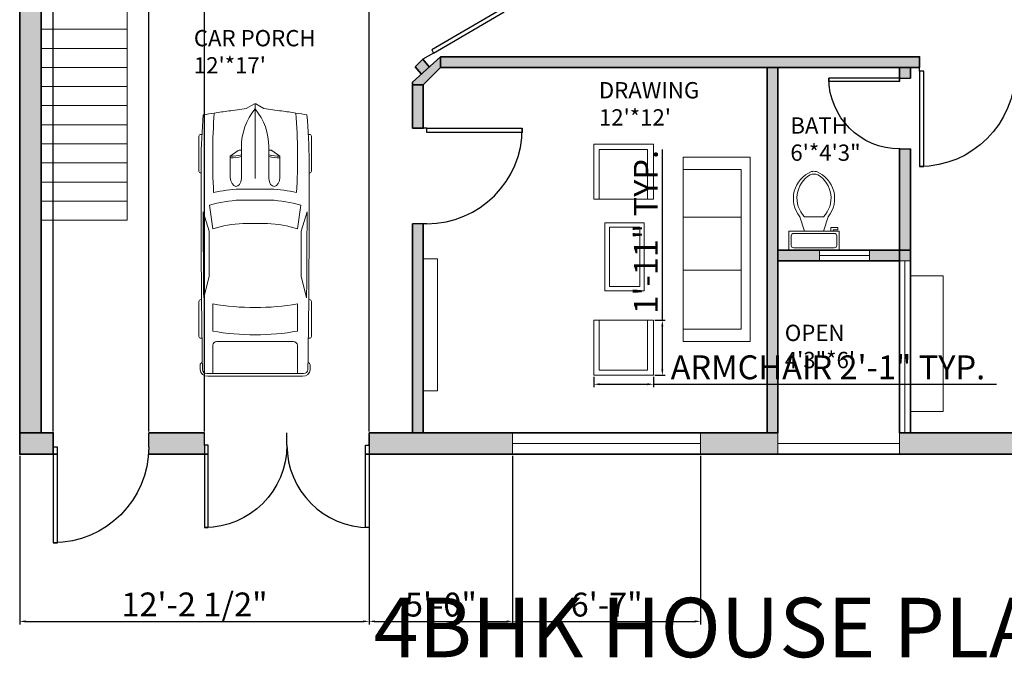
# Model space of a CAD drawing. Units: inches. Extents: x 1433 to 2137, y 2961 to 3626.
# Tile 1 of 3: x 1487 to 1899, y 2961 to 3228. Entities that reach past the tile are written whole.
import ezdxf

# ---------------------------------------------------------------- set-up
doc = ezdxf.new("R2010")
doc.units = ezdxf.units.IN
for name, color, linetype, lineweight in [('A-ANNO-DIMS', 2, 'Continuous', 18), ('A-ANNO-TEXT', 7, 'Continuous', 25), ('A-AREA-IDEN', 7, 'Continuous', 18), ('A-EQPM-VEHI', 8, 'Continuous', 13), ('A-FLOR-FIXT', 9, 'Continuous', 18), ('A-FLOR-STRS', 7, 'Continuous', 18), ('A-FURN', 8, 'Continuous', 18), ('A-WALL-PATT', 46, 'Continuous', 13), ('door', 50, 'Continuous', 25), ('wall', 46, 'Continuous', 35), ('window', 30, 'Continuous', 18)]:
    doc.layers.add(name, color=color, linetype=linetype, lineweight=lineweight)
doc.styles.get("Standard").update_dxf_attribs({"font": 'arial.ttf'})
doc.dimstyles.new('ISO-25', dxfattribs={"dimtxt": 10, "dimasz": 2.5, "dimexe": 1.25, "dimexo": 0.625, "dimtad": 1, "dimdec": 0, "dimlunit": 4, "dimtxsty": 'Standard', "dimcen": 2.5, "dimadec": 0, "dimazin": 0, "dimtfac": 1, "dimtdec": 0, "dimtmove": 0, "dimatfit": 3, "dimfxl": 1, "dimarcsym": 0})

# ---------------------------------------------------------------- blocks, each defined once
blk = doc.blocks.new('*U2')
for p, q in [((0, 0), (0, -6)), ((40, 0), (40, -6))]:
    blk.add_line(p, q)
blk.add_lwpolyline([(0, 0), (0, 40), (1.75, 40), (1.75, 0)], close=True)
blk.add_arc((0, 0), 40, 0, 90)
blk = doc.blocks.new('*U4')
for p, q in [((9.5, -6), (9.5, -2)), ((-8, -8.5), (-8, -8)), ((-7, -8), (-7, -9.5)), ((-4, -8), (-6, -14)), ((4, -8), (6, -14)), ((-10, -8.5), (-8, -8.5)), ((-10, -9.5), (-10, -8.5)), ((-7, -9.5), (-10, -9.5)), ((4, -14), (-4, -14))]:
    blk.add_line(p, q)
blk.add_lwpolyline([(10.5, -8), (10.5, 0), (-10.5, 0), (-10.5, -8)], close=True)
for points in [[(-9.5, -2), (-9.5, -6)], [(8.5, -1), (-8.5, -1)], [(-8.5, -7), (8.5, -7)]]:
    blk.add_lwpolyline(points)
for centre, radius, start, end in [((-8.62, -1.88), 0.884, 81.8699, 188.1301), ((8.62, -1.88), 0.884, 351.8699, 98.1301), ((-8.62, -6.12), 0.884, 171.8699, 278.1301), ((8.62, -6.12), 0.884, 261.8699, 8.1301), ((3.52, -21.58), 12.17, 141.4691, 247.9714), ((4.2, -21.82), 11.33, 136.3677, 238.9468), ((-3.52, -21.58), 12.17, 292.0284, 38.5307), ((-4.2, -21.82), 11.33, 301.053, 43.6321), ((0, -27.88), 4, 245.7318, 294.2682), ((0, -29), 4, 254.8605, 285.1395)]:
    blk.add_arc(centre, radius, start, end)
blk = doc.blocks.new('*U6')
for p, q in [((21.1, 37.41), (21.1, 36.83)), ((46.55, 38.89), (22.35, 38.89)), ((47.8, 37.39), (47.8, 37.41)), ((87.99, 31.87), (74.76, 35.92)), ((134.31, 35.6), (119.29, 31.78)), ((135.45, 37.07), (135.45, 37.41)), ((136.7, 38.89), (160.9, 38.89)), ((162.15, 37.41), (162.15, 36.77)), ((70.03, 31.54), (86.41, 29.35)), ((138.42, 29.35), (157.25, 29.35)), ((186.47, 29.35), (167.01, 29.35)), ((186.47, -33.5), (186.47, 33.5)), ((188.4, -32.76), (188.4, 32.76)), ((164.52, 26.39), (164.52, -26.39)), ((32.27, 11.63), (36.13, 17.17)), ((36.13, 17.17), (50.94, 17.17)), ((29.77, 9.51), (51.68, 9.51)), ((32.12, 9.51), (32.12, 11.15)), ((58.92, -10.77), (58.92, 10.77)), ((66.55, -10.53), (66.55, 10.53)), ((82.74, 8.5), (82.74, -8.5)), ((186.47, -10.53), (186.47, 10.53)), ((3.27, 6.13), (0.1, 0.41)), ((0, 0), (51.68, 0)), ((0.1, -0.41), (3.27, -6.13)), ((29.77, -9.51), (51.68, -9.51)), ((32.12, -9.51), (32.12, -11.15)), ((32.27, -11.63), (36.13, -17.17)), ((36.13, -17.17), (50.94, -17.17)), ((86.41, -29.35), (70.03, -31.54)), ((87.99, -31.87), (74.76, -35.92)), ((134.31, -35.6), (119.29, -31.78)), ((157.25, -29.35), (138.42, -29.35)), ((167.01, -29.35), (186.47, -29.35)), ((21.1, -37.41), (21.1, -36.83)), ((46.55, -38.89), (22.35, -38.89)), ((47.8, -37.39), (47.8, -37.41)), ((135.45, -37.07), (135.45, -37.41)), ((136.7, -38.89), (160.9, -38.89)), ((162.15, -37.41), (162.15, -36.77))]:
    blk.add_line(p, q)
for centre, major_axis, ratio, start_param, end_param in [((266.03, -27.52), (0, 313.31), 0.842304, 1.367076, 1.39176), ((41.19, -490.86), (0, 528.23), 0.842304, 0.00281, 0.075598), ((22.35, 37.41), (0, -1.48), 0.842304, 3.141593, 4.712389), ((64.48, -10555.62), (0, 10593.03), 0.842304, -0.013397, 0.002797), ((46.55, 37.41), (0, 1.48), 0.842304, -1.570796, 0), ((64.48, -10555.62), (0, -10591.55), 0.842304, 3.133765, 3.140441), ((136.7, 37.41), (0, -1.48), 0.842304, 3.141593, 4.712389), ((160.9, 37.41), (0, 1.48), 0.842304, -1.570796, 0), ((180.63, 35.84), (0, 2.22), 0.842304, -0.013017, 1.249894), ((64.48, -10556.36), (0, 10595.31), 0.842304, -0.013397, -0.013017), ((183.98, 33.5), (0, -2.96), 0.842304, 1.570796, 3.128196), ((183.98, 32.76), (0, -5.25), 0.842304, 1.570796, 3.128196), ((259.18, -27.52), (0, -305.3), 0.842304, 4.528606, 4.561838), ((37.47, -593.96), (0, -623.33), 0.842304, 3.096046, 3.200911), ((134.4, 5.39), (0, -89.78), 0.842304, 4.449482, 4.652344), ((135.29, 5.39), (0, 81.77), 0.842304, 1.245306, 1.50788), ((149.6, 2.8), (0, -79.58), 0.842304, 4.372215, 4.640744), ((95.79, -3666.35), (0, -3698.24), 0.842304, 3.134049, 3.144098), ((17.08, 0), (0, 147.02), 0.842304, 4.511394, 4.913384), ((35.91, 0), (0, 147.02), 0.842304, 4.511394, 4.913384), ((167.01, 26.39), (0, 2.96), 0.842304, 0, 1.570796), ((-204.49, 52.4), (0, -250.96), 0.842304, 1.385369, 1.434372), ((13.04, 17.01), (0, 27.42), 0.842304, 4.435146, 4.718221), ((14.2, 17.01), (0, 27.42), 0.842304, 4.435146, 4.718221), ((50.79, 13.34), (6.34, -0.36), 0.603834, -1.395552, 1.581315), ((29.77, -46.66), (0, 56.17), 0.842304, 0, 0.590319), ((32.75, 11.15), (0, 0.74), 0.842304, 0.879714, 1.570796), ((0.62, 0), (0, -0.74), 0.842304, 4.131459, 5.293319), ((-204.49, -52.4), (0, 250.96), 0.842304, -1.434372, -1.385369), ((29.77, 46.66), (0, 56.17), 0.842304, 2.551274, 3.141593), ((32.75, -11.15), (0, -0.74), 0.842304, 4.712389, 5.403472), ((13.04, -17.01), (0, -27.42), 0.842304, 1.564964, 1.848039), ((14.2, -17.01), (0, -27.42), 0.842304, 1.564964, 1.848039), ((134.4, -5.39), (0, -89.78), 0.842304, -1.510751, -1.307889), ((135.29, -5.39), (0, -81.77), 0.842304, -1.50788, -1.245306), ((149.6, -2.8), (0, -79.58), 0.842304, -1.499151, -1.230623), ((259.18, 27.52), (0, 305.3), 0.842304, 1.721348, 1.754579), ((167.01, -26.39), (0, -2.96), 0.842304, 4.712389, 6.283185), ((266.03, 27.52), (0, 313.31), 0.842304, 1.749832, 1.774517), ((37.47, 593.96), (0, -623.33), 0.842304, -0.059319, 0.045547), ((95.79, 3666.35), (0, -3698.24), 0.842304, -0.002505, 0.007544), ((183.98, -33.5), (0, 2.96), 0.842304, 3.15499, 4.712389), ((183.98, -32.76), (0, -5.25), 0.842304, 0.013397, 1.570796), ((41.19, 490.86), (0, -528.23), 0.842304, -0.075598, -0.00281), ((22.35, -37.41), (0, 1.48), 0.842304, 1.570796, 3.141593), ((64.48, 10555.62), (0, 10593.03), 0.842304, 3.138796, 3.15499), ((46.55, -37.41), (0, -1.48), 0.842304, 0, 1.570796), ((64.48, 10555.62), (0, -10591.55), 0.842304, 0.001152, 0.007828), ((136.7, -37.41), (0, -1.48), 0.842304, -1.570796, 0), ((160.9, -37.41), (0, 1.48), 0.842304, 3.141593, 4.712389), ((180.63, -35.84), (0, -2.22), 0.842304, -1.249894, 0.013017), ((64.48, 10556.36), (0, 10595.31), 0.842304, 3.15461, 3.15499)]:
    blk.add_ellipse(centre, major_axis=major_axis, ratio=ratio, start_param=start_param, end_param=end_param)
at = {"extrusion": (0, 0, -1)}
blk.add_ellipse((50.79, -13.34), major_axis=(6.34, 0.36), ratio=0.603834, start_param=-1.395552, end_param=1.581315, dxfattribs=at)
blk = doc.blocks.new('ARMCHAIR-COMPACT')
for p, q in [((0, 0), (0, 23.05)), ((0, 23.05), (2.27, 23.05)), ((22.52, 23.05), (24.95, 23.05)), ((24.95, 23.05), (24.95, 0)), ((24.95, 0), (0, 0))]:
    blk.add_line(p, q)
blk.add_lwpolyline([(22.52, 23.05), (2.27, 23.05), (2.27, 2.22), (22.52, 2.22)], close=True)
blk = doc.blocks.new('*D20')
at = {"layer": 'A-ANNO-DIMS', "color": 0, "lineweight": -2, "transparency": 16777216}
for p, q in [((1727.19, 3078.76), (1727.19, 3074.39)), ((1752.14, 3078.76), (1752.14, 3074.39)), ((1729.69, 3075.64), (1749.64, 3075.64)), ((1752.14, 3075.64), (1895.82, 3075.64))]:
    blk.add_line(p, q, dxfattribs=at)
at = {"layer": 'A-ANNO-DIMS', "color": 0, "transparency": 16777216}
for points in [[(1729.69, 3076.06), (1729.69, 3075.22), (1727.19, 3075.64)], [(1749.64, 3076.06), (1749.64, 3075.22), (1752.14, 3075.64)]]:
    blk.add_solid(points, dxfattribs=at)
at = {"layer": 'Defpoints', "color": 0, "transparency": 16777216}
for p in [(1727.19, 3079.38), (1752.14, 3079.38), (1752.14, 3075.64)]:
    blk.add_point(p, dxfattribs=at)
at = {"layer": 'A-ANNO-DIMS', "color": 0, "transparency": 16777216, "insert": (1825.23, 3081.44), "char_height": 10, "attachment_point": 5}
blk.add_mtext('ARMCHAIR 2\'-1" TYP.', dxfattribs=at)
blk = doc.blocks.new('*D21')
at = {"layer": 'A-ANNO-DIMS', "color": 0, "lineweight": -2, "transparency": 16777216}
for p, q in [((1755.88, 3102.43), (1755.88, 3173.96)), ((1752.77, 3102.43), (1757.13, 3102.43)), ((1755.88, 3081.88), (1755.88, 3099.93)), ((1752.77, 3079.38), (1757.13, 3079.38))]:
    blk.add_line(p, q, dxfattribs=at)
at = {"layer": 'A-ANNO-DIMS', "color": 0, "transparency": 16777216}
for points in [[(1755.47, 3099.93), (1756.3, 3099.93), (1755.88, 3102.43)], [(1755.47, 3081.88), (1756.3, 3081.88), (1755.88, 3079.38)]]:
    blk.add_solid(points, dxfattribs=at)
at = {"layer": 'Defpoints', "color": 0, "transparency": 16777216}
for p in [(1752.14, 3102.43), (1755.88, 3102.43), (1752.14, 3079.38)]:
    blk.add_point(p, dxfattribs=at)
at = {"layer": 'A-ANNO-DIMS', "color": 0, "transparency": 16777216, "insert": (1750.24, 3139.45), "char_height": 10, "attachment_point": 5, "rotation": 90}
blk.add_mtext('1\'-11" TYP.', dxfattribs=at)
blk = doc.blocks.new('*D33')
at = {"layer": 'A-ANNO-DIMS', "color": 0, "lineweight": -2, "transparency": 16777216}
for p, q in [((1633.11, 3054.67), (1633.11, 2975.1)), ((1486.74, 3045.67), (1486.74, 2975.1)), ((1489.24, 2976.35), (1630.61, 2976.35))]:
    blk.add_line(p, q, dxfattribs=at)
at = {"layer": 'A-ANNO-DIMS', "color": 0, "transparency": 16777216}
for points in [[(1489.24, 2976.76), (1489.24, 2975.93), (1486.74, 2976.35)], [(1630.61, 2976.76), (1630.61, 2975.93), (1633.11, 2976.35)]]:
    blk.add_solid(points, dxfattribs=at)
at = {"layer": 'Defpoints', "color": 0, "transparency": 16777216}
for p in [(1633.11, 3055.3), (1486.74, 3046.3), (1633.11, 2976.35)]:
    blk.add_point(p, dxfattribs=at)
at = {"layer": 'A-ANNO-DIMS', "color": 0, "transparency": 16777216, "insert": (1559.93, 2982.14), "char_height": 10, "attachment_point": 5}
blk.add_mtext('12\'-2 1/2"', dxfattribs=at)
blk = doc.blocks.new('*D34')
at = {"layer": 'A-ANNO-DIMS', "color": 0, "lineweight": -2, "transparency": 16777216}
for p, q in [((1500.78, 3055.92), (1500.78, 3560.5)), ((1503.28, 3559.25), (1538.28, 3559.25)), ((1540.78, 3055.92), (1540.78, 3560.5))]:
    blk.add_line(p, q, dxfattribs=at)
at = {"layer": 'A-ANNO-DIMS', "color": 0, "transparency": 16777216}
for points in [[(1503.28, 3559.66), (1503.28, 3558.83), (1500.78, 3559.25)], [(1538.28, 3559.66), (1538.28, 3558.83), (1540.78, 3559.25)]]:
    blk.add_solid(points, dxfattribs=at)
at = {"layer": 'Defpoints', "color": 0, "transparency": 16777216}
for p in [(1540.78, 3559.25), (1500.78, 3055.3), (1540.78, 3055.3)]:
    blk.add_point(p, dxfattribs=at)
at = {"layer": 'A-ANNO-DIMS', "color": 0, "transparency": 16777216, "insert": (1520.78, 3564.98), "char_height": 10, "attachment_point": 5}
blk.add_mtext('3\'-4"', dxfattribs=at)
blk = doc.blocks.new('*D35')
at = {"layer": 'A-ANNO-DIMS', "color": 0, "lineweight": -2, "transparency": 16777216}
for p, q in [((1540.78, 3055.92), (1540.78, 3560.5)), ((1543.28, 3559.25), (1561.69, 3559.25)), ((1564.19, 3055.92), (1564.19, 3560.5)), ((1564.19, 3559.25), (1624.66, 3559.25))]:
    blk.add_line(p, q, dxfattribs=at)
at = {"layer": 'A-ANNO-DIMS', "color": 0, "transparency": 16777216}
for points in [[(1543.28, 3559.66), (1543.28, 3558.83), (1540.78, 3559.25)], [(1561.69, 3559.66), (1561.69, 3558.83), (1564.19, 3559.25)]]:
    blk.add_solid(points, dxfattribs=at)
at = {"layer": 'Defpoints', "color": 0, "transparency": 16777216}
for p in [(1564.19, 3559.25), (1540.78, 3055.3), (1564.19, 3055.3)]:
    blk.add_point(p, dxfattribs=at)
at = {"layer": 'A-ANNO-DIMS', "color": 0, "transparency": 16777216, "insert": (1595.68, 3565.04), "char_height": 10, "attachment_point": 5}
blk.add_mtext('1\'-11 1/2"', dxfattribs=at)
blk = doc.blocks.new('*D36')
at = {"layer": 'A-ANNO-DIMS', "color": 0, "lineweight": -2, "transparency": 16777216}
for p, q in [((1564.19, 3055.92), (1564.19, 3560.5)), ((1566.69, 3559.25), (1630.61, 3559.25)), ((1633.11, 3055.92), (1633.11, 3560.5))]:
    blk.add_line(p, q, dxfattribs=at)
at = {"layer": 'A-ANNO-DIMS', "color": 0, "transparency": 16777216}
for points in [[(1566.69, 3559.66), (1566.69, 3558.83), (1564.19, 3559.25)], [(1630.61, 3559.66), (1630.61, 3558.83), (1633.11, 3559.25)]]:
    blk.add_solid(points, dxfattribs=at)
at = {"layer": 'Defpoints', "color": 0, "transparency": 16777216}
for p in [(1633.11, 3559.25), (1564.19, 3055.3), (1633.11, 3055.3)]:
    blk.add_point(p, dxfattribs=at)
at = {"layer": 'A-ANNO-DIMS', "color": 0, "transparency": 16777216, "insert": (1598.65, 3564.98), "char_height": 10, "attachment_point": 5}
blk.add_mtext('5\'-9"', dxfattribs=at)
blk = doc.blocks.new('*D37')
at = {"layer": 'A-ANNO-DIMS', "color": 0, "lineweight": -2, "transparency": 16777216}
for p, q in [((1633.11, 3054.67), (1633.11, 2975.1)), ((1693.15, 3045.67), (1693.15, 2975.1)), ((1635.61, 2976.35), (1690.65, 2976.35))]:
    blk.add_line(p, q, dxfattribs=at)
at = {"layer": 'A-ANNO-DIMS', "color": 0, "transparency": 16777216}
for points in [[(1635.61, 2976.76), (1635.61, 2975.93), (1633.11, 2976.35)], [(1690.65, 2976.76), (1690.65, 2975.93), (1693.15, 2976.35)]]:
    blk.add_solid(points, dxfattribs=at)
at = {"layer": 'Defpoints', "color": 0, "transparency": 16777216}
for p in [(1633.11, 3055.3), (1693.15, 3046.3), (1693.15, 2976.35)]:
    blk.add_point(p, dxfattribs=at)
at = {"layer": 'A-ANNO-DIMS', "color": 0, "transparency": 16777216, "insert": (1663.13, 2982.08), "char_height": 10, "attachment_point": 5}
blk.add_mtext('5\'-0"', dxfattribs=at)
blk = doc.blocks.new('*D38')
at = {"layer": 'A-ANNO-DIMS', "color": 0, "lineweight": -2, "transparency": 16777216}
for p, q in [((1693.15, 3045.67), (1693.15, 2975.1)), ((1771.92, 3045.67), (1771.92, 2975.1)), ((1695.65, 2976.35), (1769.42, 2976.35))]:
    blk.add_line(p, q, dxfattribs=at)
at = {"layer": 'A-ANNO-DIMS', "color": 0, "transparency": 16777216}
for points in [[(1695.65, 2976.76), (1695.65, 2975.93), (1693.15, 2976.35)], [(1769.42, 2976.76), (1769.42, 2975.93), (1771.92, 2976.35)]]:
    blk.add_solid(points, dxfattribs=at)
at = {"layer": 'Defpoints', "color": 0, "transparency": 16777216}
for p in [(1693.15, 3046.3), (1771.92, 3046.3), (1771.92, 2976.35)]:
    blk.add_point(p, dxfattribs=at)
at = {"layer": 'A-ANNO-DIMS', "color": 0, "transparency": 16777216, "insert": (1732.54, 2982.08), "char_height": 10, "attachment_point": 5}
blk.add_mtext('6\'-7"', dxfattribs=at)

msp = doc.modelspace()

# ---------------------------------------------------------------- hatches: boundary and pattern name
at = {"layer": 'A-WALL-PATT'}
h = msp.add_hatch(color=256, dxfattribs=at)
h.dxf.hatch_style = 1
h.paths.add_polyline_path([(1684.74, 3517.3), (1675.74, 3517.3), (1675.74, 3405.93), (1679.92, 3405.93, -0.043454), (1684.74, 3405.51)])
h.paths.add_polyline_path([(1861.24, 3373.3), (1801.24, 3373.3), (1801.24, 3439.3), (1861.24, 3439.3), (1861.24, 3443.8), (1796.74, 3443.8), (1796.74, 3368.8), (1861.24, 3368.8)])
h.paths.add_polyline_path([(1749.24, 3443.8), (1684.74, 3443.8), (1684.74, 3439.3), (1744.74, 3439.3), (1744.74, 3373.3), (1684.74, 3373.3), (1684.74, 3368.8), (1749.24, 3368.8)])
h.paths.add_polyline_path([(1684.74, 3378.05), (1679.92, 3378.05), (1675.74, 3378.05), (1675.74, 3373.3), (1672.64, 3373.3), (1672.64, 3368.8), (1684.74, 3368.8), (1684.74, 3373.3)])
h.paths.add_polyline_path([(1865.74, 3378.26), (1861.56, 3378.26), (1861.24, 3378.26), (1861.24, 3368.8), (1869.81, 3368.8), (1869.81, 3373.3), (1865.74, 3373.3)])
h.paths.add_polyline_path([(2057.74, 3373.3), (1909.81, 3373.3), (1909.81, 3368.8), (2057.74, 3368.8)])
h.paths.add_polyline_path([(1919.74, 3368.8), (1915.24, 3368.8), (1915.24, 3366.92), (1919.74, 3366.92)])
h.paths.add_polyline_path([(1919.74, 3326.92), (1915.24, 3326.92), (1915.24, 3308.14), (1919.74, 3308.14)])
h.paths.add_polyline_path([(1919.74, 3236.84), (1915.24, 3236.84), (1915.24, 3212.8), (1919.74, 3212.8)])
h.paths.add_polyline_path([(1859.74, 3208.3), (1855.24, 3208.3), (1855.24, 3203.85), (1855.29, 3203.85), (1859.74, 3203.85)])
h = msp.add_hatch(color=256, dxfattribs=at)
h.dxf.hatch_style = 1
h.paths.add_polyline_path([(1500.78, 3055.3), (1486.74, 3055.3), (1486.74, 3046.3), (1500.78, 3046.3), (1500.78, 3049.3)])
h.paths.add_polyline_path([(1495.74, 3412.16), (1486.74, 3412.16), (1486.74, 3055.3), (1495.74, 3055.3)])
h = msp.add_hatch(color=256, dxfattribs=at)
h.dxf.hatch_style = 1
h.paths.add_polyline_path([(1632.64, 3373.3), (1495.74, 3373.3), (1495.74, 3368.8), (1632.64, 3368.8)])
h.paths.add_polyline_path([(1620.24, 3368.8), (1615.74, 3368.8), (1615.74, 3362.47), (1620.24, 3362.47)])
h.paths.add_polyline_path([(1526.85, 3272.8), (1495.74, 3272.8), (1495.74, 3268.3), (1526.85, 3268.3)])
h.paths.add_polyline_path([(1612.35, 3272.8), (1579.17, 3272.8), (1579.17, 3268.3), (1607.43, 3268.3), (1608.56, 3269.33)])
h.paths.add_polyline_path([(1620.24, 3275.2), (1620.24, 3280), (1608.56, 3269.33), (1607.43, 3268.3), (1613.07, 3268.3)])
h.paths.add_polyline_path([(1620.24, 3322.47), (1615.74, 3322.47), (1615.74, 3275.89), (1620.24, 3280)])
h.paths.add_polyline_path([(1621.12, 3270.32), (1618.48, 3273.5), (1615.2, 3270.34), (1617.74, 3267.34)])
h.paths.add_polyline_path([(1658.27, 3208.55), (1655.63, 3211.74), (1652.35, 3208.58), (1654.95, 3205.51)])
h.paths.add_polyline_path([(1564.19, 3050.13), (1564.19, 3055.3), (1540.78, 3055.3), (1540.78, 3049.3, -0.01877), (1540.67, 3046.3), (1564.19, 3046.3)])
h.paths.add_polyline_path([(1693.15, 3055.3), (1655.74, 3055.3), (1633.11, 3055.3), (1633.11, 3050.13), (1633.11, 3046.3), (1693.15, 3046.3)])
h.paths.add_polyline_path([(1804.24, 3127.3), (1804.24, 3208.3), (1799.74, 3208.3), (1799.74, 3131.8), (1799.74, 3055.3), (1804.24, 3055.3)])
h.paths.add_polyline_path([(1655.74, 3142.86), (1651.24, 3142.86), (1651.24, 3055.3), (1655.74, 3055.3)])
h.paths.add_polyline_path([(2057.74, 3212.8), (1903.59, 3212.8), (1903.59, 3208.3), (2057.74, 3208.3)])
h.paths.add_polyline_path([(1855.24, 3055.3), (1855.24, 3046.3), (2066.74, 3046.3), (2066.74, 3094.86), (2057.74, 3094.86), (2057.74, 3094.45), (2057.74, 3071.77), (2057.74, 3055.3)])
h = msp.add_hatch(color=256, dxfattribs=at)
h.dxf.hatch_style = 1
h.paths.add_polyline_path([(1863.59, 3212.8), (1662.92, 3212.8), (1662.92, 3208.3), (1863.59, 3208.3)])
h.paths.add_polyline_path([(1662.92, 3212.8), (1651.24, 3202.12), (1651.24, 3201.08), (1655.74, 3201.08), (1662.92, 3208.3)])
h.paths.add_polyline_path([(1655.74, 3201.08), (1651.24, 3201.08), (1651.24, 3182.86), (1655.74, 3182.86)])
h.paths.add_polyline_path([(1859.74, 3174.18), (1855.24, 3174.18), (1855.24, 3131.8), (1859.74, 3131.8)])
h.paths.add_polyline_path([(1859.74, 3131.8), (1855.24, 3131.8), (1855.24, 3127.3), (1859.74, 3127.3)])
h.paths.add_polyline_path([(1855.24, 3131.8), (1842.62, 3131.8), (1842.62, 3127.3), (1855.24, 3127.3)])
h.paths.add_polyline_path([(1821.69, 3131.8), (1808.89, 3131.8), (1804.24, 3131.8), (1804.24, 3127.3), (1821.69, 3127.3)])
h = msp.add_hatch(color=256, dxfattribs=at)
h.dxf.hatch_style = 1
h.paths.add_polyline_path([(1804.24, 3055.3), (1771.92, 3055.3), (1771.92, 3046.3), (1804.24, 3046.3)])

# ---------------------------------------------------------------- linework, layer by layer
at = {"layer": 'A-FLOR-STRS'}
for p, q in [((1531.74, 3144.3), (1531.74, 3232.3)), ((1531.74, 3224.3), (1495.74, 3224.3)), ((1531.74, 3216.3), (1495.74, 3216.3)), ((1531.74, 3208.3), (1495.74, 3208.3)), ((1531.74, 3200.3), (1495.74, 3200.3)), ((1531.74, 3192.3), (1495.74, 3192.3)), ((1531.74, 3184.3), (1495.74, 3184.3)), ((1531.74, 3176.3), (1495.74, 3176.3)), ((1531.74, 3168.3), (1495.74, 3168.3)), ((1531.74, 3160.3), (1495.74, 3160.3)), ((1531.74, 3152.3), (1495.74, 3152.3)), ((1531.74, 3144.3), (1495.74, 3144.3))]:
    msp.add_line(p, q, dxfattribs=at)
at = {"layer": 'A-FURN'}
for p, q in [((1764.61, 3165.63), (1764.61, 3170.75)), ((1764.61, 3170.75), (1792.71, 3170.75)), ((1792.71, 3170.75), (1792.71, 3170.75)), ((1792.71, 3170.75), (1792.71, 3093.52)), ((1788.85, 3145.63), (1764.61, 3145.63)), ((1788.85, 3123.39), (1764.61, 3123.39)), ((1764.61, 3093.52), (1764.61, 3103.55)), ((1792.71, 3093.52), (1764.61, 3093.52))]:
    msp.add_line(p, q, dxfattribs=at)
for points in [[(1788.85, 3165.63), (1764.61, 3165.63), (1764.61, 3098.72), (1788.85, 3098.72)], [(1731.86, 3143.24), (1748.31, 3143.24), (1748.31, 3114.7), (1731.86, 3114.7)], [(1733.7, 3141.4), (1746.47, 3141.4), (1746.47, 3116.54), (1733.7, 3116.54)], [(1655.74, 3128.19), (1661.68, 3128.19), (1661.68, 3072.93), (1655.74, 3072.93)], [(1859.74, 3064.3), (1873.45, 3064.3), (1873.45, 3121.06), (1859.74, 3121.06)]]:
    msp.add_lwpolyline(points, close=True, dxfattribs=at)
at = {"layer": 'wall'}
for p, q in [((1486.74, 3046.3), (1486.74, 3526.3)), ((1495.74, 3055.3), (1495.74, 3517.3)), ((1651.24, 3202.12), (1662.92, 3212.8)), ((1651.24, 3202.12), (1662.92, 3212.8)), ((1799.74, 3212.8), (1662.92, 3212.8)), ((1799.74, 3212.8), (1863.59, 3212.8)), ((1863.59, 3212.8), (1855.24, 3212.8)), ((1652.35, 3208.58), (1655.63, 3211.74)), ((1652.35, 3208.58), (1654.9, 3205.58)), ((1658.27, 3208.55), (1655.63, 3211.74)), ((1655.74, 3201.08), (1662.92, 3208.3)), ((1804.24, 3208.3), (1663.23, 3208.3)), ((1799.74, 3131.8), (1799.74, 3208.3)), ((1804.24, 3127.3), (1804.24, 3208.3)), ((1859.74, 3208.3), (1804.24, 3208.3)), ((1855.24, 3208.3), (1855.24, 3202.56)), ((1859.74, 3208.3), (1859.74, 3203.85)), ((1863.59, 3208.3), (1859.74, 3208.3)), ((1654.9, 3205.58), (1654.95, 3205.51)), ((1651.24, 3182.86), (1651.24, 3202.12)), ((1651.24, 3201.08), (1651.24, 3202.12)), ((1655.74, 3199.3), (1655.74, 3201.08)), ((1655.74, 3182.86), (1655.74, 3201.08)), ((1855.24, 3131.8), (1855.24, 3174.18)), ((1855.24, 3174.18), (1855.24, 3064.3)), ((1859.74, 3174.18), (1859.74, 3064.3)), ((1651.24, 3055.3), (1651.24, 3142.86)), ((1655.74, 3055.3), (1655.74, 3142.86)), ((1799.74, 3055.3), (1799.74, 3131.8)), ((1804.24, 3131.8), (1855.24, 3131.8)), ((1855.24, 3131.8), (1859.74, 3131.8)), ((1804.24, 3055.3), (1804.24, 3127.3)), ((1804.24, 3127.3), (1855.24, 3127.3)), ((1855.24, 3064.3), (1855.24, 3055.3)), ((1859.74, 3064.3), (1859.74, 3055.3)), ((1500.78, 3055.3), (1495.74, 3055.3)), ((1564.19, 3055.3), (1540.78, 3055.3)), ((1804.24, 3055.3), (1633.11, 3055.3)), ((1799.74, 3055.3), (1655.74, 3055.3)), ((2057.74, 3055.3), (1855.24, 3055.3)), ((1502.53, 3046.3), (1486.74, 3046.3)), ((1565.7, 3046.3), (1540.67, 3046.3)), ((1598.87, 3046.3), (1598.44, 3046.3)), ((2066.74, 3046.3), (1631.6, 3046.3))]:
    msp.add_line(p, q, dxfattribs=at)
for points in [[(1486.74, 3412.16), (1495.74, 3412.16), (1495.74, 3055.3), (1486.74, 3055.3)], [(1662.92, 3212.8), (1863.59, 3212.8), (1863.59, 3208.3), (1662.92, 3208.3)], [(1651.24, 3182.86), (1655.74, 3182.86), (1655.74, 3201.08), (1651.24, 3201.08)], [(1651.24, 3201.08), (1655.74, 3201.08), (1655.74, 3201.08), (1651.24, 3201.08)], [(1500.78, 3046.3), (1486.74, 3046.3), (1486.74, 3055.3), (1500.78, 3055.3)]]:
    msp.add_lwpolyline(points, close=True, dxfattribs=at)
at = {"layer": 'window'}
for p, q in [((1821.69, 3129.55), (1842.62, 3129.55)), ((1857.49, 3127.3), (1857.49, 3055.3)), ((1804.24, 3055.3), (1804.24, 3046.3)), ((1855.24, 3055.3), (1855.24, 3046.3)), ((1693.15, 3050.8), (1771.92, 3050.8)), ((1855.24, 3050.8), (1804.24, 3050.8))]:
    msp.add_line(p, q, dxfattribs=at)
for points in [[(1821.69, 3131.8), (1842.62, 3131.8), (1842.62, 3127.3), (1821.69, 3127.3)], [(1855.24, 3127.3), (1859.74, 3127.3), (1859.74, 3055.3), (1855.24, 3055.3)], [(1693.15, 3055.3), (1771.92, 3055.3), (1771.92, 3046.3), (1693.15, 3046.3)]]:
    msp.add_lwpolyline(points, close=True, dxfattribs=at)

# ---------------------------------------------------------------- block references
at = {"layer": 'A-EQPM-VEHI', "xscale": 0.6052825972638168, "yscale": 0.6052825972638168, "zscale": 0.6052825972638168, "rotation": 270}
msp.add_blockref('*U6', (1585.34, 3193.06), dxfattribs=at)
at = {"layer": 'A-FLOR-FIXT', "rotation": 180}
msp.add_blockref('*U4', (1819.39, 3131.8), dxfattribs=at)
at = {"layer": 'A-FURN', "extrusion": (0, 0, -1), "zscale": -1, "rotation": 180}
msp.add_blockref('ARMCHAIR-COMPACT', (-1727.19, 3176.19), dxfattribs=at)
at = {"layer": 'A-FURN'}
msp.add_blockref('ARMCHAIR-COMPACT', (1727.19, 3079.38), dxfattribs=at)
at = {"layer": 'door'}
for p, xscale, yscale, zscale, rotation in [((1660.06, 3214.32), -0.8544553422168171, 0.8544553422168171, 0.8544553422168168, 300.2802112171161), ((1855.29, 3203.85), -0.7418126355599052, 0.7418126355599052, 0.7418126355599052, 90), ((1564.19, 3050.13), -0.8614770298831453, 0.8614770298831453, 0.8614770298831453, 180), ((1633.11, 3050.13), 0.8614770298831453, 0.8614770298831453, 0.8614770298831453, 180)]:
    msp.add_blockref('*U2', p, dxfattribs=dict(at, xscale=xscale, yscale=yscale, zscale=zscale, rotation=rotation))
at = {"layer": 'door', "xscale": -1, "rotation": 180}
for p in [(1863.59, 3206.8), (1500.78, 3049.3)]:
    msp.add_blockref('*U2', p, dxfattribs=at)
at = {"layer": 'door', "rotation": 270}
msp.add_blockref('*U2', (1657.24, 3182.86), dxfattribs=at)

# ---------------------------------------------------------------- texts
at = {"layer": 'A-ANNO-TEXT', "insert": (1634.97, 2986.23), "char_height": 24.8992, "attachment_point": 1}
msp.add_mtext_dynamic_manual_height_columns('4BHK HOUSE PLAN', width=495.0792, gutter_width=124.5, heights=[0], dxfattribs=at)
at = {"layer": 'A-AREA-IDEN', "char_height": 6.823, "attachment_point": 1}
for s, insert in [("CAR PORCH\\P12'*17'", (1559.67, 3223.98)), ("DRAWING\\P12'*12'", (1729.31, 3202.17)), ('BATH\\P6\'*4\'3"', (1809.49, 3187.4)), ('OPEN\\P4\'3"*6\'', (1807.15, 3100.57))]:
    msp.add_mtext_dynamic_manual_height_columns(s, width=135.668, gutter_width=34.12, heights=[0], dxfattribs=dict(at, insert=insert))

# ---------------------------------------------------------------- dimensions: what is measured, and where the dimension line sits
at = {"layer": 'A-ANNO-DIMS'}
for base, p1, p2, picture, middle in [((1564.19, 3559.25), (1540.78, 3055.3), (1564.19, 3055.3), '*D35', (1595.68, 3565.04)), ((1540.78, 3559.25), (1500.78, 3055.3), (1540.78, 3055.3), '*D34', (1520.78, 3564.98)), ((1633.11, 3559.25), (1564.19, 3055.3), (1633.11, 3055.3), '*D36', (1598.65, 3564.98)), ((1633.11, 2976.35), (1486.74, 3046.3), (1633.11, 3055.3), '*D33', (1559.93, 2982.14)), ((1693.15, 2976.35), (1633.11, 3055.3), (1693.15, 3046.3), '*D37', (1663.13, 2982.08)), ((1771.92, 2976.35), (1693.15, 3046.3), (1771.92, 3046.3), '*D38', (1732.54, 2982.08))]:
    dim = msp.add_linear_dim(base=base, p1=p1, p2=p2, dimstyle='ISO-25', override={"dimdec": 1, "dimlfac": 1, "dimrnd": 0, "dimzin": 1, "dimdsep": 46, "dimlunit": 4, "dimfrac": 2}, dxfattribs=at)
    dim.commit()
    dim.dimension.update_dxf_attribs({"geometry": picture, "text_midpoint": middle})
dim = msp.add_linear_dim(base=(1755.884, 3102.429), p1=(1752.1411, 3079.3839), p2=(1752.1411, 3102.429), angle=90, text='<> TYP.', dimstyle='ISO-25', override={"dimdec": 1, "dimlfac": 1, "dimrnd": 0, "dimzin": 1, "dimdsep": 46, "dimlunit": 4, "dimfrac": 2}, dxfattribs=at)
dim.commit()
dim.dimension.update_dxf_attribs({"geometry": '*D21', "text_midpoint": (1750.2352, 3139.4456)})
dim = msp.add_linear_dim(base=(1752.1411, 3075.641), p1=(1727.1883, 3079.3839), p2=(1752.1411, 3079.3839), text='ARMCHAIR <> TYP.', dimstyle='ISO-25', override={"dimdec": 1, "dimlfac": 1, "dimrnd": 0, "dimzin": 1, "dimdsep": 46, "dimlunit": 4, "dimfrac": 2}, dxfattribs=at)
dim.commit()
dim.dimension.update_dxf_attribs({"geometry": '*D20', "text_midpoint": (1825.2286, 3081.4365)})

doc.saveas('drawing.dxf')
